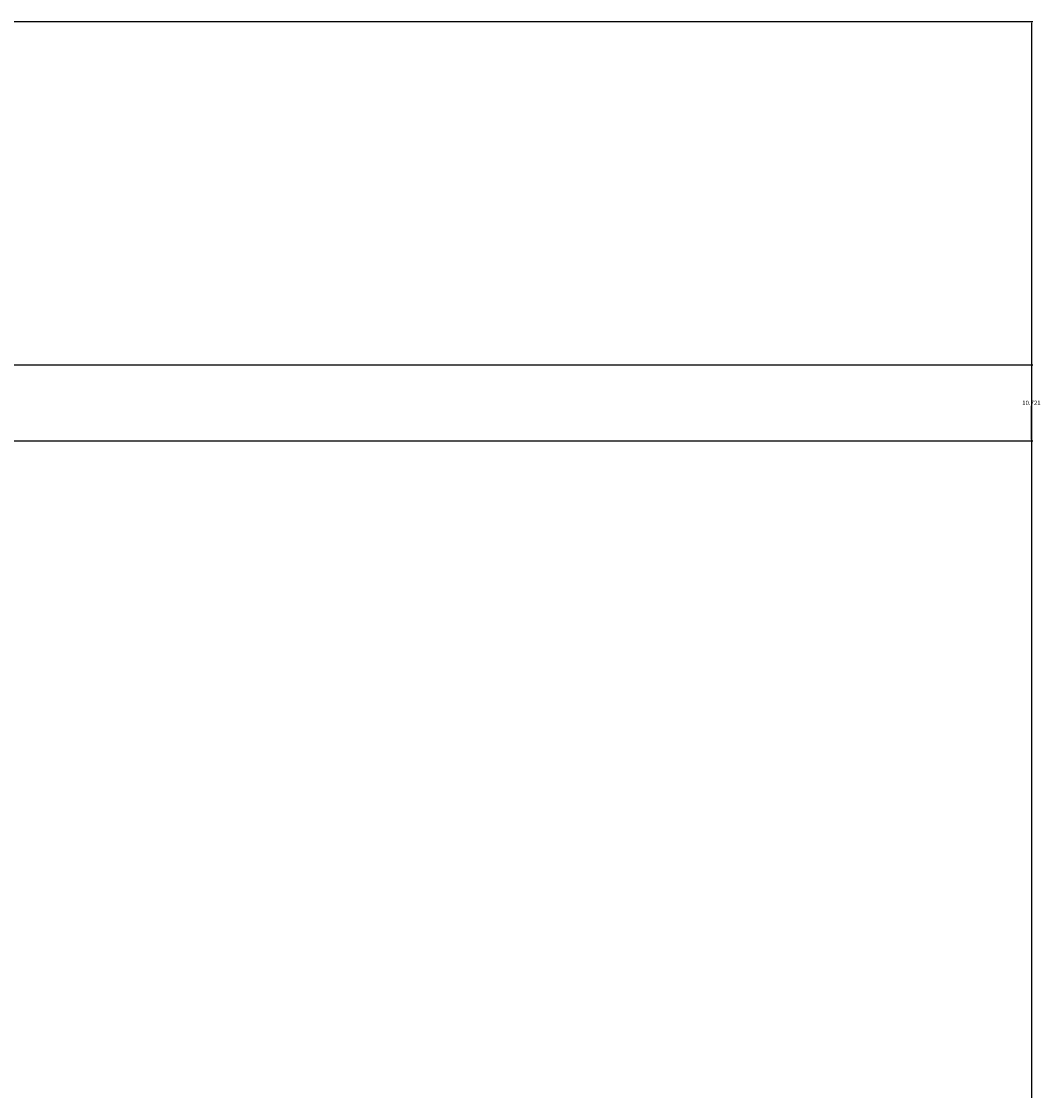
# Model space of a CAD drawing. Units: inches. Extents: x -13 to 809, y 112 to 656.
# Tile 55 of 55: x 665 to 809, y 467 to 618. Entities that reach past the tile are written whole.
import ezdxf

# ---------------------------------------------------------------- set-up
doc = ezdxf.new("R2010")
doc.units = ezdxf.units.IN
doc.header["$MEASUREMENT"] = 0
doc.layers.add('A-ANNO-DIMS', color=2, linetype='Continuous', lineweight=18)
doc.styles.get("Standard").update_dxf_attribs({"font": 'arial.ttf'})
doc.dimstyles.get("Standard").update_dxf_attribs({"dimtxt": 0.625, "dimasz": 0.18, "dimexe": 0.18, "dimexo": 0.0625, "dimgap": 0.09, "dimtad": 0, "dimtih": 1, "dimtoh": 1, "dimdec": 4, "dimzin": 0, "dimdsep": 46, "dimlunit": 4, "dimtxsty": 'Standard', "dimcen": 0.09, "dimadec": 0, "dimazin": 0, "dimtfac": 1, "dimtdec": 4, "dimtofl": 0, "dimtmove": 0, "dimatfit": 3, "dimfxl": 1, "dimtolj": 1, "dimtzin": 0, "dimarcsym": 0})

# ---------------------------------------------------------------- blocks, each defined once
blk = doc.blocks.new('*D31')
at = {"layer": 'A-ANNO-DIMS', "color": 0, "lineweight": -2, "transparency": 16777216}
for p, q in [((621.07, 617.78), (807.77, 617.78)), ((807.59, 617.6), (807.59, 384.56)), ((807.59, 150.7), (807.59, 383.74)), ((621.07, 150.52), (807.77, 150.52))]:
    blk.add_line(p, q, dxfattribs=at)
at = {"layer": 'A-ANNO-DIMS', "color": 0, "transparency": 16777216}
for points in [[(807.56, 617.6), (807.62, 617.6), (807.59, 617.78)], [(807.56, 150.7), (807.62, 150.7), (807.59, 150.52)]]:
    blk.add_solid(points, dxfattribs=at)
at = {"layer": 'Defpoints', "color": 0, "transparency": 16777216}
for p in [(621.01, 617.78), (807.59, 617.78), (621.01, 150.52)]:
    blk.add_point(p, dxfattribs=at)
at = {"layer": 'A-ANNO-DIMS', "color": 0, "transparency": 16777216, "insert": (807.59, 384.15), "char_height": 0.625, "attachment_point": 5}
blk.add_mtext('\\A1;467.3', dxfattribs=at)
blk = doc.blocks.new('*D38')
at = {"layer": 'A-ANNO-DIMS', "color": 0, "lineweight": -2, "transparency": 16777216}
for p, q in [((644.68, 569.24), (807.77, 569.24)), ((807.59, 569.06), (807.59, 564.29)), ((807.59, 558.7), (807.59, 563.47)), ((644.68, 558.52), (807.77, 558.52))]:
    blk.add_line(p, q, dxfattribs=at)
at = {"layer": 'A-ANNO-DIMS', "color": 0, "transparency": 16777216}
for points in [[(807.56, 569.06), (807.62, 569.06), (807.59, 569.24)], [(807.56, 558.7), (807.62, 558.7), (807.59, 558.52)]]:
    blk.add_solid(points, dxfattribs=at)
at = {"layer": 'Defpoints', "color": 0, "transparency": 16777216}
for p in [(644.62, 569.24), (807.59, 569.24), (644.62, 558.52)]:
    blk.add_point(p, dxfattribs=at)
at = {"layer": 'A-ANNO-DIMS', "color": 0, "transparency": 16777216, "insert": (807.59, 563.88), "char_height": 0.625, "attachment_point": 5}
blk.add_mtext('\\A1;10.721', dxfattribs=at)

msp = doc.modelspace()

# ---------------------------------------------------------------- dimensions: what is measured, and where the dimension line sits
at = {"layer": 'A-ANNO-DIMS'}
for base, p1, p2, override, picture, middle in [((807.5888, 617.7828), (621.008, 150.5199), (621.008, 617.7828), {"dimdec": 1, "dimlfac": 1, "dimrnd": 0, "dimzin": 0, "dimdsep": 46, "dimlunit": 2}, '*D31', (807.5888, 384.1514)), ((807.588831, 569.241385), (644.622094, 558.519894), (644.622094, 569.241385), {"dimdec": 3, "dimlfac": 1, "dimrnd": 0, "dimzin": 0, "dimdsep": 46, "dimlunit": 2}, '*D38', (807.588831, 563.88064))]:
    dim = msp.add_linear_dim(base=base, p1=p1, p2=p2, angle=90, dimstyle='Standard', override=override, dxfattribs=at)
    dim.commit()
    dim.dimension.update_dxf_attribs({"geometry": picture, "text_midpoint": middle})

doc.saveas('drawing.dxf')
